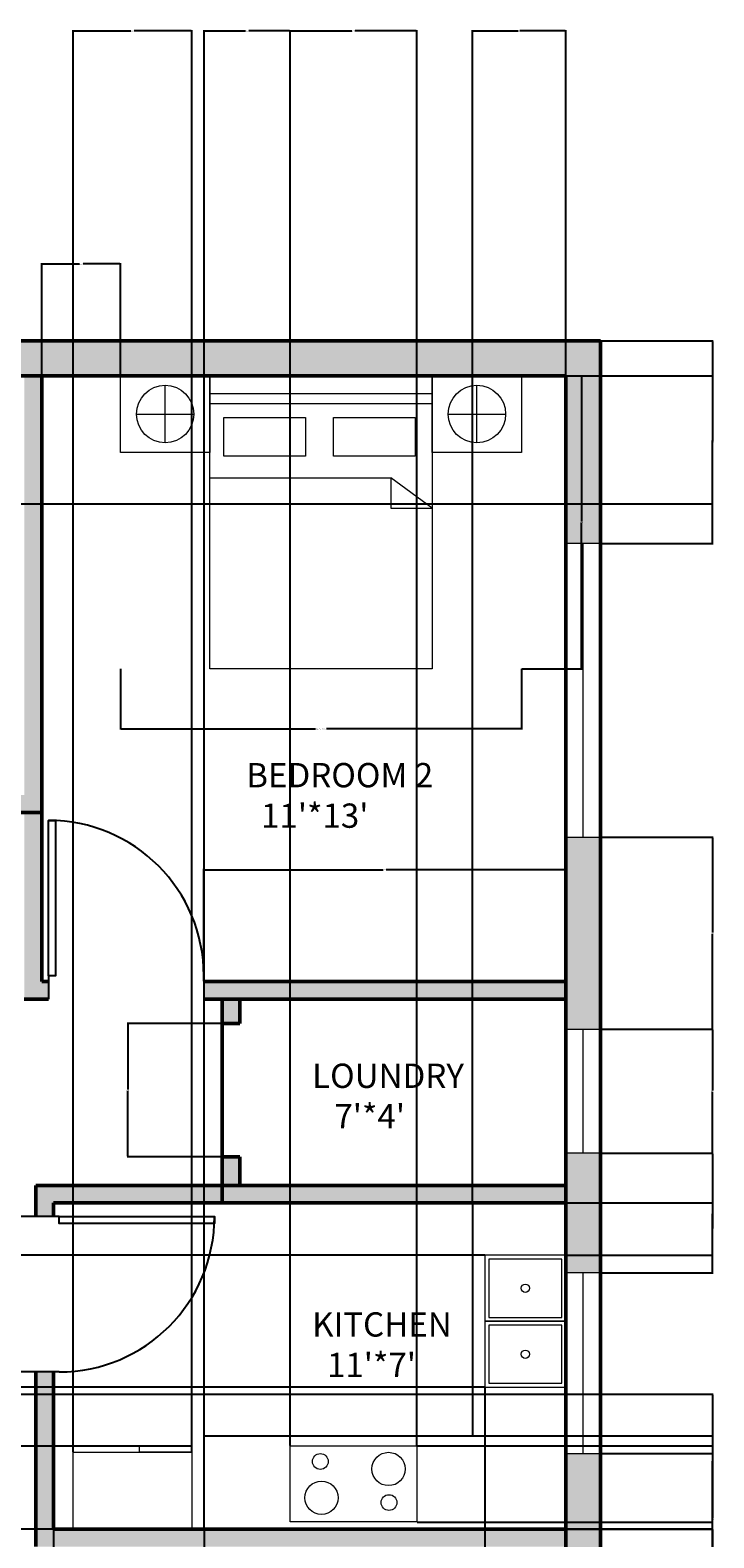
# Model space of a CAD drawing. Units: inches. Extents: x 2405 to 2823, y 1214 to 1813.
# Tile 4 of 4: x 2647 to 2823, y 1425 to 1813. Entities that reach past the tile are written whole.
import ezdxf

# ---------------------------------------------------------------- set-up
doc = ezdxf.new("R2010")
doc.units = ezdxf.units.IN
for name, color, linetype, lineweight in [('A-ANNO-DIMS', 2, 'Continuous', 18), ('A-AREA-IDEN', 30, 'Continuous', 25), ('A-EQPM', 8, 'Continuous', 18), ('A-FLOR-CASE', 8, 'Continuous', 25), ('A-FLOR-FIXT', 9, 'Continuous', 18), ('A-WALL-PATT', 252, 'Continuous', 13), ('DOOR', 133, 'Continuous', 25), ('FUR', 10, 'Continuous', 18), ('WALL', 140, 'Continuous', 50), ('WIND', 200, 'Continuous', 18)]:
    doc.layers.add(name, color=color, linetype=linetype, lineweight=lineweight)
doc.styles.get("Standard").update_dxf_attribs({"font": 'arial.ttf'})
doc.dimstyles.get("Standard").update_dxf_attribs({"dimtxt": 0.18, "dimasz": 0.18, "dimexe": 0.18, "dimexo": 0.0625, "dimgap": 0.09, "dimtad": 0, "dimtih": 1, "dimtoh": 1, "dimdec": 4, "dimzin": 0, "dimdsep": 46, "dimtxsty": 'Standard', "dimcen": 0.09, "dimadec": 0, "dimazin": 0, "dimtfac": 1, "dimtdec": 4, "dimtofl": 0, "dimtmove": 0, "dimatfit": 3, "dimfxl": 1, "dimtolj": 1, "dimtzin": 0, "dimarcsym": 0})

# ---------------------------------------------------------------- blocks, each defined once
blk = doc.blocks.new('*U2')
for p, q in [((0, 0), (0, -6)), ((40, 0), (40, -6))]:
    blk.add_line(p, q)
blk.add_lwpolyline([(0, 0), (0, 40), (1.75, 40), (1.75, 0)], close=True)
blk.add_arc((0, 0), 40, 0, 90)
blk = doc.blocks.new('BED-DOUBLE-WITH-NIGHTSTANDS')
for p, q in [((11.49, 58.17), (11.49, 72.97)), ((91.81, 58.17), (91.81, 72.97)), ((4.09, 65.57), (18.88, 65.57)), ((84.41, 65.57), (99.2, 65.57)), ((22.97, 49.14), (69.63, 49.14)), ((69.63, 49.14), (69.63, 41.32)), ((80.32, 41.32), (69.63, 49.14)), ((69.63, 41.32), (80.32, 41.32))]:
    blk.add_line(p, q)
for points in [[(0, 75.45), (22.97, 75.45), (22.97, 55.69), (0, 55.69)], [(22.97, 75.45), (80.32, 75.45), (80.32, 0), (22.97, 0)], [(80.32, 75.45), (103.29, 75.45), (103.29, 55.69), (80.32, 55.69)], [(22.97, 70.85), (80.32, 70.85), (80.32, 68.18), (22.97, 68.18)], [(26.59, 64.68), (47.64, 64.68), (47.64, 54.75), (26.59, 54.75)], [(54.85, 64.68), (75.89, 64.68), (75.89, 54.75), (54.85, 54.75)]]:
    blk.add_lwpolyline(points, close=True)
for centre in [(11.49, 65.57), (91.81, 65.57)]:
    blk.add_circle(centre, 7.4)
blk = doc.blocks.new('WIN-75_625')
blk.add_line((4.5, 0), (4.5, 75.63))
blk.add_lwpolyline([(9, 75.63), (0, 75.63), (0, 0), (9, 0)], close=True)
blk = doc.blocks.new('WIN-46_53')
blk.add_line((4.5, 0), (4.5, 46.53))
blk.add_lwpolyline([(0, 0), (9, 0), (9, 46.53), (0, 46.53)], close=True)
blk = doc.blocks.new('*D16')
at = {"layer": 'A-ANNO-DIMS', "color": 0, "lineweight": -2, "transparency": 16777216}
for p, q in [((2670.07, 1648.42), (2670.07, 1632.81)), ((2773.36, 1648.42), (2773.36, 1632.81)), ((2670.25, 1632.99), (2720.34, 1632.99)), ((2773.18, 1632.99), (2723.1, 1632.99))]:
    blk.add_line(p, q, dxfattribs=at)
at = {"layer": 'A-ANNO-DIMS', "color": 0, "lineweight": 100, "transparency": 16777216}
for points in [[(2670.25, 1633.02), (2670.25, 1632.96), (2670.07, 1632.99)], [(2773.18, 1633.02), (2773.18, 1632.96), (2773.36, 1632.99)]]:
    blk.add_solid(points, dxfattribs=at)
at = {"layer": 'Defpoints', "color": 0, "lineweight": 100, "transparency": 16777216}
for p in [(2670.07, 1648.48), (2773.36, 1648.48), (2773.36, 1632.99)]:
    blk.add_point(p, dxfattribs=at)
at = {"layer": 'A-ANNO-DIMS', "color": 0, "transparency": 16777216, "insert": (2721.72, 1632.99), "char_height": 0.18, "attachment_point": 5}
blk.add_mtext('\\A1;BED GROUP 103 TYP.', dxfattribs=at)
blk = doc.blocks.new('*D17')
at = {"layer": 'A-ANNO-DIMS', "color": 0, "lineweight": -2, "transparency": 16777216}
for p, q in [((2773.43, 1723.93), (2789.04, 1723.93)), ((2788.86, 1723.75), (2788.86, 1686.39)), ((2788.86, 1648.66), (2788.86, 1686.02)), ((2773.43, 1648.48), (2789.04, 1648.48))]:
    blk.add_line(p, q, dxfattribs=at)
at = {"layer": 'A-ANNO-DIMS', "color": 0, "lineweight": 100, "transparency": 16777216}
for points in [[(2788.83, 1723.75), (2788.89, 1723.75), (2788.86, 1723.93)], [(2788.83, 1648.66), (2788.89, 1648.66), (2788.86, 1648.48)]]:
    blk.add_solid(points, dxfattribs=at)
at = {"layer": 'Defpoints', "color": 0, "lineweight": 100, "transparency": 16777216}
for p in [(2773.36, 1723.93), (2788.86, 1723.93), (2773.36, 1648.48)]:
    blk.add_point(p, dxfattribs=at)
at = {"layer": 'A-ANNO-DIMS', "color": 0, "transparency": 16777216, "insert": (2788.86, 1686.21), "char_height": 0.18, "attachment_point": 5}
blk.add_mtext('\\A1;75 TYP.', dxfattribs=at)
blk = doc.blocks.new('*D24')
at = {"layer": 'A-ANNO-DIMS', "color": 0, "lineweight": -2, "transparency": 16777216}
for p, q in [((2793.83, 1732.93), (2822.75, 1732.93)), ((2822.57, 1732.75), (2822.57, 1707.02)), ((2822.57, 1680.92), (2822.57, 1706.65)), ((2793.83, 1680.74), (2822.75, 1680.74))]:
    blk.add_line(p, q, dxfattribs=at)
at = {"layer": 'A-ANNO-DIMS', "color": 0, "lineweight": 100, "transparency": 16777216}
for points in [[(2822.54, 1732.75), (2822.6, 1732.75), (2822.57, 1732.93)], [(2822.54, 1680.92), (2822.6, 1680.92), (2822.57, 1680.74)]]:
    blk.add_solid(points, dxfattribs=at)
at = {"layer": 'Defpoints', "color": 0, "lineweight": 100, "transparency": 16777216}
for p in [(2793.77, 1732.93), (2793.77, 1680.74), (2822.57, 1680.74)]:
    blk.add_point(p, dxfattribs=at)
at = {"layer": 'A-ANNO-DIMS', "color": 0, "transparency": 16777216, "insert": (2822.57, 1706.83), "char_height": 0.18, "attachment_point": 5}
blk.add_mtext('\\A1;52.19', dxfattribs=at)
blk = doc.blocks.new('*D26')
at = {"layer": 'A-ANNO-DIMS', "color": 0, "lineweight": -2, "transparency": 16777216}
for p, q in [((2793.83, 1605.11), (2822.75, 1605.11)), ((2822.57, 1604.93), (2822.57, 1580.57)), ((2822.57, 1555.85), (2822.57, 1580.21)), ((2793.83, 1555.67), (2822.75, 1555.67))]:
    blk.add_line(p, q, dxfattribs=at)
at = {"layer": 'A-ANNO-DIMS', "color": 0, "lineweight": 100, "transparency": 16777216}
for points in [[(2822.54, 1604.93), (2822.6, 1604.93), (2822.57, 1605.11)], [(2822.54, 1555.85), (2822.6, 1555.85), (2822.57, 1555.67)]]:
    blk.add_solid(points, dxfattribs=at)
at = {"layer": 'Defpoints', "color": 0, "lineweight": 100, "transparency": 16777216}
for p in [(2793.77, 1605.11), (2793.77, 1555.67), (2822.57, 1555.67)]:
    blk.add_point(p, dxfattribs=at)
at = {"layer": 'A-ANNO-DIMS', "color": 0, "transparency": 16777216, "insert": (2822.57, 1580.39), "char_height": 0.18, "attachment_point": 5}
blk.add_mtext('\\A1;49.44', dxfattribs=at)
blk = doc.blocks.new('*D27')
at = {"layer": 'A-ANNO-DIMS', "color": 0, "lineweight": -2, "transparency": 16777216}
for p, q in [((2793.83, 1555.67), (2822.75, 1555.67)), ((2822.57, 1555.49), (2822.57, 1539.88)), ((2822.57, 1523.92), (2822.57, 1539.52)), ((2793.83, 1523.74), (2822.75, 1523.74))]:
    blk.add_line(p, q, dxfattribs=at)
at = {"layer": 'A-ANNO-DIMS', "color": 0, "lineweight": 100, "transparency": 16777216}
for points in [[(2822.54, 1555.49), (2822.6, 1555.49), (2822.57, 1555.67)], [(2822.54, 1523.92), (2822.6, 1523.92), (2822.57, 1523.74)]]:
    blk.add_solid(points, dxfattribs=at)
at = {"layer": 'Defpoints', "color": 0, "lineweight": 100, "transparency": 16777216}
for p in [(2793.77, 1555.67), (2793.77, 1523.74), (2822.57, 1523.74)]:
    blk.add_point(p, dxfattribs=at)
at = {"layer": 'A-ANNO-DIMS', "color": 0, "transparency": 16777216, "insert": (2822.57, 1539.7), "char_height": 0.18, "attachment_point": 5}
blk.add_mtext('\\A1;31.93', dxfattribs=at)
blk = doc.blocks.new('*D28')
at = {"layer": 'A-ANNO-DIMS', "color": 0, "lineweight": -2, "transparency": 16777216}
for p, q in [((2793.83, 1523.74), (2822.75, 1523.74)), ((2822.57, 1523.56), (2822.57, 1508.52)), ((2822.57, 1493.11), (2822.57, 1508.15)), ((2793.83, 1492.93), (2822.75, 1492.93))]:
    blk.add_line(p, q, dxfattribs=at)
at = {"layer": 'A-ANNO-DIMS', "color": 0, "lineweight": 100, "transparency": 16777216}
for points in [[(2822.54, 1523.56), (2822.6, 1523.56), (2822.57, 1523.74)], [(2822.54, 1493.11), (2822.6, 1493.11), (2822.57, 1492.93)]]:
    blk.add_solid(points, dxfattribs=at)
at = {"layer": 'Defpoints', "color": 0, "lineweight": 100, "transparency": 16777216}
for p in [(2793.77, 1523.74), (2793.77, 1492.93), (2822.57, 1492.93)]:
    blk.add_point(p, dxfattribs=at)
at = {"layer": 'A-ANNO-DIMS', "color": 0, "transparency": 16777216, "insert": (2822.57, 1508.33), "char_height": 0.18, "attachment_point": 5}
blk.add_mtext('\\A1;30.807', dxfattribs=at)
blk = doc.blocks.new('*D29')
at = {"layer": 'A-ANNO-DIMS', "color": 0, "lineweight": -2, "transparency": 16777216}
for p, q in [((2793.83, 1446.4), (2822.75, 1446.4)), ((2822.57, 1446.22), (2822.57, 1429.71)), ((2822.57, 1412.83), (2822.57, 1429.35)), ((2793.83, 1412.65), (2822.75, 1412.65))]:
    blk.add_line(p, q, dxfattribs=at)
at = {"layer": 'A-ANNO-DIMS', "color": 0, "lineweight": 100, "transparency": 16777216}
for points in [[(2822.54, 1446.22), (2822.6, 1446.22), (2822.57, 1446.4)], [(2822.54, 1412.83), (2822.6, 1412.83), (2822.57, 1412.65)]]:
    blk.add_solid(points, dxfattribs=at)
at = {"layer": 'Defpoints', "color": 0, "lineweight": 100, "transparency": 16777216}
for p in [(2793.77, 1446.4), (2793.77, 1412.65), (2822.57, 1412.65)]:
    blk.add_point(p, dxfattribs=at)
at = {"layer": 'A-ANNO-DIMS', "color": 0, "transparency": 16777216, "insert": (2822.57, 1429.53), "char_height": 0.18, "attachment_point": 5}
blk.add_mtext('\\A1;33.754', dxfattribs=at)
blk = doc.blocks.new('*D38')
at = {"layer": 'A-ANNO-DIMS', "color": 0, "lineweight": -2, "transparency": 16777216}
for p, q in [((2760.77, 1510.99), (2760.77, 1812.91)), ((2760.95, 1812.73), (2772.55, 1812.73)), ((2784.59, 1812.73), (2772.99, 1812.73)), ((2784.77, 1510.99), (2784.77, 1812.91))]:
    blk.add_line(p, q, dxfattribs=at)
at = {"layer": 'A-ANNO-DIMS', "color": 0, "lineweight": 100, "transparency": 16777216}
for points in [[(2760.95, 1812.76), (2760.95, 1812.7), (2760.77, 1812.73)], [(2784.59, 1812.76), (2784.59, 1812.7), (2784.77, 1812.73)]]:
    blk.add_solid(points, dxfattribs=at)
at = {"layer": 'Defpoints', "color": 0, "lineweight": 100, "transparency": 16777216}
for p in [(2760.77, 1812.73), (2760.77, 1510.93), (2784.77, 1510.93)]:
    blk.add_point(p, dxfattribs=at)
at = {"layer": 'A-ANNO-DIMS', "color": 0, "transparency": 16777216, "insert": (2772.77, 1812.73), "char_height": 0.18, "attachment_point": 5}
blk.add_mtext('\\A1;24', dxfattribs=at)
blk = doc.blocks.new('*D39')
at = {"layer": 'A-ANNO-DIMS', "color": 0, "lineweight": -2, "transparency": 16777216}
for p, q in [((2691.69, 1450.93), (2822.75, 1450.93)), ((2822.57, 1450.75), (2822.57, 1439.11)), ((2822.57, 1427.11), (2822.57, 1438.75)), ((2691.69, 1426.93), (2822.75, 1426.93))]:
    blk.add_line(p, q, dxfattribs=at)
at = {"layer": 'A-ANNO-DIMS', "color": 0, "lineweight": 100, "transparency": 16777216}
for points in [[(2822.54, 1450.75), (2822.6, 1450.75), (2822.57, 1450.93)], [(2822.54, 1427.11), (2822.6, 1427.11), (2822.57, 1426.93)]]:
    blk.add_solid(points, dxfattribs=at)
at = {"layer": 'Defpoints', "color": 0, "lineweight": 100, "transparency": 16777216}
for p in [(2691.63, 1450.93), (2691.63, 1426.93), (2822.57, 1426.93)]:
    blk.add_point(p, dxfattribs=at)
at = {"layer": 'A-ANNO-DIMS', "color": 0, "transparency": 16777216, "insert": (2822.57, 1438.93), "char_height": 0.18, "attachment_point": 5}
blk.add_mtext('\\A1;24', dxfattribs=at)
blk = doc.blocks.new('*D40')
at = {"layer": 'A-ANNO-DIMS', "color": 0, "lineweight": -2, "transparency": 16777216}
for p, q in [((2652.77, 1426.87), (2652.77, 1214.95)), ((2691.63, 1426.87), (2691.63, 1214.95)), ((2652.95, 1215.13), (2671.8, 1215.13)), ((2691.45, 1215.13), (2672.59, 1215.13))]:
    blk.add_line(p, q, dxfattribs=at)
at = {"layer": 'A-ANNO-DIMS', "color": 0, "lineweight": 100, "transparency": 16777216}
for points in [[(2652.95, 1215.16), (2652.95, 1215.1), (2652.77, 1215.13)], [(2691.45, 1215.16), (2691.45, 1215.1), (2691.63, 1215.13)]]:
    blk.add_solid(points, dxfattribs=at)
at = {"layer": 'Defpoints', "color": 0, "lineweight": 100, "transparency": 16777216}
for p in [(2652.77, 1426.93), (2691.63, 1426.93), (2691.63, 1215.13)]:
    blk.add_point(p, dxfattribs=at)
at = {"layer": 'A-ANNO-DIMS', "color": 0, "transparency": 16777216, "insert": (2672.2, 1215.13), "char_height": 0.18, "attachment_point": 5}
blk.add_mtext('\\A1;38.86', dxfattribs=at)
blk = doc.blocks.new('*D41')
at = {"layer": 'A-ANNO-DIMS', "color": 0, "lineweight": -2, "transparency": 16777216}
for p, q in [((2648.21, 1507.39), (2404.79, 1507.39)), ((2404.97, 1507.21), (2404.97, 1487.57)), ((2404.97, 1467.57), (2404.97, 1487.21)), ((2648.21, 1467.39), (2404.79, 1467.39))]:
    blk.add_line(p, q, dxfattribs=at)
at = {"layer": 'A-ANNO-DIMS', "color": 0, "lineweight": 100, "transparency": 16777216}
for points in [[(2404.94, 1507.21), (2405, 1507.21), (2404.97, 1507.39)], [(2404.94, 1467.57), (2405, 1467.57), (2404.97, 1467.39)]]:
    blk.add_solid(points, dxfattribs=at)
at = {"layer": 'Defpoints', "color": 0, "lineweight": 100, "transparency": 16777216}
for p in [(2648.27, 1507.39), (2404.97, 1467.39), (2648.27, 1467.39)]:
    blk.add_point(p, dxfattribs=at)
at = {"layer": 'A-ANNO-DIMS', "color": 0, "transparency": 16777216, "insert": (2404.97, 1487.39), "char_height": 0.18, "attachment_point": 5}
blk.add_mtext('\\A1;40', dxfattribs=at)
blk = doc.blocks.new('*D45')
at = {"layer": 'A-ANNO-DIMS', "color": 0, "lineweight": -2, "transparency": 16777216}
for p, q in [((2477.36, 1461.68), (2822.75, 1461.68)), ((2822.57, 1461.5), (2822.57, 1444.53)), ((2822.57, 1427.19), (2822.57, 1444.16)), ((2477.36, 1427.01), (2822.75, 1427.01))]:
    blk.add_line(p, q, dxfattribs=at)
at = {"layer": 'A-ANNO-DIMS', "color": 0, "lineweight": 100, "transparency": 16777216}
for points in [[(2822.54, 1461.5), (2822.6, 1461.5), (2822.57, 1461.68)], [(2822.54, 1427.19), (2822.6, 1427.19), (2822.57, 1427.01)]]:
    blk.add_solid(points, dxfattribs=at)
at = {"layer": 'Defpoints', "color": 0, "lineweight": 100, "transparency": 16777216}
for p in [(2477.3, 1461.68), (2477.3, 1427.01), (2822.57, 1427.01)]:
    blk.add_point(p, dxfattribs=at)
at = {"layer": 'A-ANNO-DIMS', "color": 0, "transparency": 16777216, "insert": (2822.57, 1444.34), "char_height": 0.18, "attachment_point": 5}
blk.add_mtext('\\A1;34.66', dxfattribs=at)
blk = doc.blocks.new('*D46')
at = {"layer": 'A-ANNO-DIMS', "color": 0, "lineweight": -2, "transparency": 16777216}
for p, q in [((2713.75, 1448.42), (2713.75, 1812.91)), ((2713.93, 1812.73), (2729.63, 1812.73)), ((2746.25, 1812.73), (2730.56, 1812.73)), ((2746.43, 1448.42), (2746.43, 1812.91))]:
    blk.add_line(p, q, dxfattribs=at)
at = {"layer": 'A-ANNO-DIMS', "color": 0, "lineweight": 100, "transparency": 16777216}
for points in [[(2713.93, 1812.76), (2713.93, 1812.7), (2713.75, 1812.73)], [(2746.25, 1812.76), (2746.25, 1812.7), (2746.43, 1812.73)]]:
    blk.add_solid(points, dxfattribs=at)
at = {"layer": 'Defpoints', "color": 0, "lineweight": 100, "transparency": 16777216}
for p in [(2746.43, 1812.73), (2713.75, 1448.36), (2746.43, 1448.36)]:
    blk.add_point(p, dxfattribs=at)
at = {"layer": 'A-ANNO-DIMS', "color": 0, "transparency": 16777216, "insert": (2730.09, 1812.73), "char_height": 0.18, "attachment_point": 5}
blk.add_mtext('\\A1;32.684', dxfattribs=at)
blk = doc.blocks.new('*D47')
at = {"layer": 'A-ANNO-DIMS', "color": 0, "lineweight": -2, "transparency": 16777216}
for p, q in [((2763.89, 1497.45), (2404.79, 1497.45)), ((2404.97, 1497.27), (2404.97, 1480.64)), ((2404.97, 1463.65), (2404.97, 1480.28)), ((2763.89, 1463.47), (2404.79, 1463.47))]:
    blk.add_line(p, q, dxfattribs=at)
at = {"layer": 'A-ANNO-DIMS', "color": 0, "lineweight": 100, "transparency": 16777216}
for points in [[(2404.94, 1497.27), (2405, 1497.27), (2404.97, 1497.45)], [(2404.94, 1463.65), (2405, 1463.65), (2404.97, 1463.47)]]:
    blk.add_solid(points, dxfattribs=at)
at = {"layer": 'Defpoints', "color": 0, "lineweight": 100, "transparency": 16777216}
for p in [(2763.95, 1497.45), (2404.97, 1463.47), (2763.95, 1463.47)]:
    blk.add_point(p, dxfattribs=at)
at = {"layer": 'A-ANNO-DIMS', "color": 0, "transparency": 16777216, "insert": (2404.97, 1480.46), "char_height": 0.18, "attachment_point": 5}
blk.add_mtext('\\A1;33.98', dxfattribs=at)
blk = doc.blocks.new('*D48')
at = {"layer": 'A-ANNO-DIMS', "color": 0, "lineweight": -2, "transparency": 16777216}
for p, q in [((2763.95, 1463.41), (2763.95, 1214.95)), ((2784.77, 1463.41), (2784.77, 1214.95)), ((2764.13, 1215.13), (2773.9, 1215.13)), ((2784.59, 1215.13), (2774.83, 1215.13))]:
    blk.add_line(p, q, dxfattribs=at)
at = {"layer": 'A-ANNO-DIMS', "color": 0, "lineweight": 100, "transparency": 16777216}
for points in [[(2764.13, 1215.16), (2764.13, 1215.1), (2763.95, 1215.13)], [(2784.59, 1215.16), (2784.59, 1215.1), (2784.77, 1215.13)]]:
    blk.add_solid(points, dxfattribs=at)
at = {"layer": 'Defpoints', "color": 0, "lineweight": 100, "transparency": 16777216}
for p in [(2763.95, 1463.47), (2784.77, 1463.47), (2784.77, 1215.13)]:
    blk.add_point(p, dxfattribs=at)
at = {"layer": 'A-ANNO-DIMS', "color": 0, "transparency": 16777216, "insert": (2774.36, 1215.13), "char_height": 0.18, "attachment_point": 5}
blk.add_mtext('\\A1;20.813', dxfattribs=at)
blk = doc.blocks.new('*D50')
at = {"layer": 'A-ANNO-DIMS', "color": 0, "lineweight": -2, "transparency": 16777216}
for p, q in [((2477.36, 1427.01), (2822.75, 1427.01)), ((2822.57, 1426.83), (2822.57, 1414.4)), ((2822.57, 1401.61), (2822.57, 1414.04)), ((2442.83, 1401.43), (2822.75, 1401.43))]:
    blk.add_line(p, q, dxfattribs=at)
at = {"layer": 'A-ANNO-DIMS', "color": 0, "lineweight": 100, "transparency": 16777216}
for points in [[(2822.54, 1426.83), (2822.6, 1426.83), (2822.57, 1427.01)], [(2822.54, 1401.61), (2822.6, 1401.61), (2822.57, 1401.43)]]:
    blk.add_solid(points, dxfattribs=at)
at = {"layer": 'Defpoints', "color": 0, "lineweight": 100, "transparency": 16777216}
for p in [(2477.3, 1427.01), (2822.57, 1427.01), (2442.77, 1401.43)]:
    blk.add_point(p, dxfattribs=at)
at = {"layer": 'A-ANNO-DIMS', "color": 0, "transparency": 16777216, "insert": (2822.57, 1414.22), "char_height": 0.18, "attachment_point": 5}
blk.add_mtext('\\A1;25.584', dxfattribs=at)
blk = doc.blocks.new('*D51')
at = {"layer": 'A-ANNO-DIMS', "color": 0, "lineweight": -2, "transparency": 16777216}
for p, q in [((2746.5, 1448.36), (2822.75, 1448.36)), ((2822.57, 1448.18), (2822.57, 1438.74)), ((2822.57, 1428.94), (2822.57, 1438.38)), ((2746.5, 1428.76), (2822.75, 1428.76))]:
    blk.add_line(p, q, dxfattribs=at)
at = {"layer": 'A-ANNO-DIMS', "color": 0, "lineweight": 100, "transparency": 16777216}
for points in [[(2822.54, 1448.18), (2822.6, 1448.18), (2822.57, 1448.36)], [(2822.54, 1428.94), (2822.6, 1428.94), (2822.57, 1428.76)]]:
    blk.add_solid(points, dxfattribs=at)
at = {"layer": 'Defpoints', "color": 0, "lineweight": 100, "transparency": 16777216}
for p in [(2746.43, 1448.36), (2746.43, 1428.76), (2822.57, 1428.76)]:
    blk.add_point(p, dxfattribs=at)
at = {"layer": 'A-ANNO-DIMS', "color": 0, "transparency": 16777216, "insert": (2822.57, 1438.56), "char_height": 0.18, "attachment_point": 5}
blk.add_mtext('\\A1;19.593', dxfattribs=at)
blk = doc.blocks.new('*D53')
at = {"layer": 'A-ANNO-DIMS', "color": 0, "lineweight": -2, "transparency": 16777216}
for p, q in [((2649.77, 1723.99), (2649.77, 1752.91)), ((2649.95, 1752.73), (2659.45, 1752.73)), ((2669.89, 1752.73), (2660.39, 1752.73)), ((2670.07, 1723.99), (2670.07, 1752.91))]:
    blk.add_line(p, q, dxfattribs=at)
at = {"layer": 'A-ANNO-DIMS', "color": 0, "lineweight": 100, "transparency": 16777216}
for points in [[(2649.95, 1752.76), (2649.95, 1752.7), (2649.77, 1752.73)], [(2669.89, 1752.76), (2669.89, 1752.7), (2670.07, 1752.73)]]:
    blk.add_solid(points, dxfattribs=at)
at = {"layer": 'Defpoints', "color": 0, "lineweight": 100, "transparency": 16777216}
for p in [(2670.07, 1752.73), (2649.77, 1723.93), (2670.07, 1723.93)]:
    blk.add_point(p, dxfattribs=at)
at = {"layer": 'A-ANNO-DIMS', "color": 0, "transparency": 16777216, "insert": (2659.92, 1752.73), "char_height": 0.18, "attachment_point": 5}
blk.add_mtext('\\A1;20.305', dxfattribs=at)
blk = doc.blocks.new('*D55')
at = {"layer": 'A-ANNO-DIMS', "color": 0, "lineweight": -2, "transparency": 16777216}
for p, q in [((2700.71, 1557.1), (2671.79, 1557.1)), ((2671.97, 1556.92), (2671.97, 1540.13)), ((2671.97, 1522.97), (2671.97, 1539.77)), ((2700.71, 1522.79), (2671.79, 1522.79))]:
    blk.add_line(p, q, dxfattribs=at)
at = {"layer": 'A-ANNO-DIMS', "color": 0, "lineweight": 100, "transparency": 16777216}
for points in [[(2671.94, 1556.92), (2672, 1556.92), (2671.97, 1557.1)], [(2671.94, 1522.97), (2672, 1522.97), (2671.97, 1522.79)]]:
    blk.add_solid(points, dxfattribs=at)
at = {"layer": 'Defpoints', "color": 0, "lineweight": 100, "transparency": 16777216}
for p in [(2671.97, 1557.1), (2700.77, 1557.1), (2700.77, 1522.79)]:
    blk.add_point(p, dxfattribs=at)
at = {"layer": 'A-ANNO-DIMS', "color": 0, "transparency": 16777216, "insert": (2671.97, 1539.95), "char_height": 0.18, "attachment_point": 5}
blk.add_mtext('\\A1;34.31', dxfattribs=at)
blk = doc.blocks.new('*D57')
at = {"layer": 'A-ANNO-DIMS', "color": 0, "lineweight": -2, "transparency": 16777216}
for p, q in [((2622.83, 1723.93), (2822.75, 1723.93)), ((2822.57, 1723.75), (2822.57, 1707.61)), ((2822.57, 1691.11), (2822.57, 1707.25)), ((2612.33, 1690.93), (2822.75, 1690.93))]:
    blk.add_line(p, q, dxfattribs=at)
at = {"layer": 'A-ANNO-DIMS', "color": 0, "lineweight": 100, "transparency": 16777216}
for points in [[(2822.54, 1723.75), (2822.6, 1723.75), (2822.57, 1723.93)], [(2822.54, 1691.11), (2822.6, 1691.11), (2822.57, 1690.93)]]:
    blk.add_solid(points, dxfattribs=at)
at = {"layer": 'Defpoints', "color": 0, "lineweight": 100, "transparency": 16777216}
for p in [(2622.77, 1723.93), (2612.27, 1690.93), (2822.57, 1690.93)]:
    blk.add_point(p, dxfattribs=at)
at = {"layer": 'A-ANNO-DIMS', "color": 0, "transparency": 16777216, "insert": (2822.57, 1707.43), "char_height": 0.18, "attachment_point": 5}
blk.add_mtext('\\A1;33', dxfattribs=at)
blk = doc.blocks.new('*D58')
at = {"layer": 'A-ANNO-DIMS', "color": 0, "lineweight": -2, "transparency": 16777216}
for p, q in [((2691.63, 1450.99), (2691.63, 1812.91)), ((2691.81, 1812.73), (2702.3, 1812.73)), ((2713.57, 1812.73), (2703.08, 1812.73)), ((2713.75, 1448.42), (2713.75, 1812.91))]:
    blk.add_line(p, q, dxfattribs=at)
at = {"layer": 'A-ANNO-DIMS', "color": 0, "lineweight": 100, "transparency": 16777216}
for points in [[(2691.81, 1812.76), (2691.81, 1812.7), (2691.63, 1812.73)], [(2713.57, 1812.76), (2713.57, 1812.7), (2713.75, 1812.73)]]:
    blk.add_solid(points, dxfattribs=at)
at = {"layer": 'Defpoints', "color": 0, "lineweight": 100, "transparency": 16777216}
for p in [(2713.75, 1812.73), (2691.63, 1450.93), (2713.75, 1448.36)]:
    blk.add_point(p, dxfattribs=at)
at = {"layer": 'A-ANNO-DIMS', "color": 0, "transparency": 16777216, "insert": (2702.69, 1812.73), "char_height": 0.18, "attachment_point": 5}
blk.add_mtext('\\A1;22.12', dxfattribs=at)
blk = doc.blocks.new('*D59')
at = {"layer": 'A-ANNO-DIMS', "color": 0, "lineweight": -2, "transparency": 16777216}
for p, q in [((2784.83, 1510.93), (2822.75, 1510.93)), ((2822.57, 1510.75), (2822.57, 1504.37)), ((2822.57, 1497.63), (2822.57, 1504.01)), ((2784.83, 1497.45), (2822.75, 1497.45))]:
    blk.add_line(p, q, dxfattribs=at)
at = {"layer": 'A-ANNO-DIMS', "color": 0, "lineweight": 100, "transparency": 16777216}
for points in [[(2822.54, 1510.75), (2822.6, 1510.75), (2822.57, 1510.93)], [(2822.54, 1497.63), (2822.6, 1497.63), (2822.57, 1497.45)]]:
    blk.add_solid(points, dxfattribs=at)
at = {"layer": 'Defpoints', "color": 0, "lineweight": 100, "transparency": 16777216}
for p in [(2784.77, 1510.93), (2822.57, 1510.93), (2784.77, 1497.45)]:
    blk.add_point(p, dxfattribs=at)
at = {"layer": 'A-ANNO-DIMS', "color": 0, "transparency": 16777216, "insert": (2822.57, 1504.19), "char_height": 0.18, "attachment_point": 5}
blk.add_mtext('\\A1;13.477', dxfattribs=at)
blk = doc.blocks.new('*D66')
at = {"layer": 'A-ANNO-DIMS', "color": 0, "lineweight": -2, "transparency": 16777216}
for p, q in [((2691.52, 1567.99), (2691.52, 1596.91)), ((2691.7, 1596.73), (2737.75, 1596.73)), ((2784.59, 1596.73), (2738.54, 1596.73)), ((2784.77, 1567.99), (2784.77, 1596.91))]:
    blk.add_line(p, q, dxfattribs=at)
at = {"layer": 'A-ANNO-DIMS', "color": 0, "lineweight": 100, "transparency": 16777216}
for points in [[(2691.7, 1596.76), (2691.7, 1596.7), (2691.52, 1596.73)], [(2784.59, 1596.76), (2784.59, 1596.7), (2784.77, 1596.73)]]:
    blk.add_solid(points, dxfattribs=at)
at = {"layer": 'Defpoints', "color": 0, "lineweight": 100, "transparency": 16777216}
for p in [(2784.77, 1596.73), (2691.52, 1567.93), (2784.77, 1567.93)]:
    blk.add_point(p, dxfattribs=at)
at = {"layer": 'A-ANNO-DIMS', "color": 0, "transparency": 16777216, "insert": (2738.14, 1596.73), "char_height": 0.18, "attachment_point": 5}
blk.add_mtext('\\A1;93.25', dxfattribs=at)
blk = doc.blocks.new('*D67')
at = {"layer": 'A-ANNO-DIMS', "color": 0, "lineweight": -2, "transparency": 16777216}
for p, q in [((2657.86, 1446.84), (2657.86, 1812.91)), ((2658.04, 1812.73), (2672.68, 1812.73)), ((2688.24, 1812.73), (2673.6, 1812.73)), ((2688.42, 1446.84), (2688.42, 1812.91))]:
    blk.add_line(p, q, dxfattribs=at)
at = {"layer": 'A-ANNO-DIMS', "color": 0, "lineweight": 100, "transparency": 16777216}
for points in [[(2658.04, 1812.76), (2658.04, 1812.7), (2657.86, 1812.73)], [(2688.24, 1812.76), (2688.24, 1812.7), (2688.42, 1812.73)]]:
    blk.add_solid(points, dxfattribs=at)
at = {"layer": 'Defpoints', "color": 0, "lineweight": 100, "transparency": 16777216}
for p in [(2688.42, 1812.73), (2657.86, 1446.78), (2688.42, 1446.78)]:
    blk.add_point(p, dxfattribs=at)
at = {"layer": 'A-ANNO-DIMS', "color": 0, "transparency": 16777216, "insert": (2673.14, 1812.73), "char_height": 0.18, "attachment_point": 5}
blk.add_mtext('\\A1;30.564', dxfattribs=at)
blk = doc.blocks.new('*D68')
at = {"layer": 'A-ANNO-DIMS', "color": 0, "lineweight": -2, "transparency": 16777216}
for p, q in [((2688.36, 1448.27), (2404.79, 1448.27)), ((2404.97, 1448.09), (2404.97, 1437.78)), ((2404.97, 1427.11), (2404.97, 1437.42)), ((2688.36, 1426.93), (2404.79, 1426.93))]:
    blk.add_line(p, q, dxfattribs=at)
at = {"layer": 'A-ANNO-DIMS', "color": 0, "lineweight": 100, "transparency": 16777216}
for points in [[(2404.94, 1448.09), (2405, 1448.09), (2404.97, 1448.27)], [(2404.94, 1427.11), (2405, 1427.11), (2404.97, 1426.93)]]:
    blk.add_solid(points, dxfattribs=at)
at = {"layer": 'Defpoints', "color": 0, "lineweight": 100, "transparency": 16777216}
for p in [(2688.42, 1448.27), (2404.97, 1426.93), (2688.42, 1426.93)]:
    blk.add_point(p, dxfattribs=at)
at = {"layer": 'A-ANNO-DIMS', "color": 0, "transparency": 16777216, "insert": (2404.97, 1437.6), "char_height": 0.18, "attachment_point": 5}
blk.add_mtext('\\A1;21.336', dxfattribs=at)

msp = doc.modelspace()

# ---------------------------------------------------------------- hatches: boundary and pattern name
at = {"layer": 'A-WALL-PATT'}
h = msp.add_hatch(color=256, dxfattribs=at)
h.dxf.hatch_style = 1
h.paths.add_polyline_path([(2601.7679, 1732.9303), (2433.7679, 1732.9303), (2433.7679, 1680.7368), (2442.7679, 1680.7368), (2442.7679, 1723.9303), (2574.7679, 1723.9303), (2601.7679, 1723.9303)])
h.paths.add_polyline_path([(2793.7679, 1732.9303), (2622.7552, 1732.9303), (2622.7552, 1723.9303), (2622.7679, 1723.9303), (2645.2679, 1723.9303), (2784.7679, 1723.9303), (2784.7679, 1680.7368), (2793.7679, 1680.7368)])
h.paths.add_polyline_path([(2442.7679, 1605.111), (2433.7679, 1605.111), (2433.7679, 1513.1454), (2442.7679, 1513.1454), (2442.7679, 1563.4303)])
h.paths.add_polyline_path([(2531.8067, 1567.9303), (2442.7679, 1567.9303), (2442.7679, 1563.4303), (2531.8067, 1563.4303)])
h.paths.add_polyline_path([(2793.7679, 1605.111), (2784.7679, 1605.111), (2784.7679, 1555.6662), (2793.7679, 1555.6662)])
h.paths.add_polyline_path([(2784.7679, 1567.9303), (2691.5187, 1567.9303), (2691.5187, 1563.4303), (2784.7679, 1563.4303)])
h.paths.add_polyline_path([(2649.7679, 1611.4303), (2645.2679, 1611.4303), (2645.2679, 1563.4303), (2651.5187, 1563.4303), (2651.5187, 1567.9303), (2649.7679, 1567.9303)])
h.paths.add_polyline_path([(2581.5295, 1614.9584), (2581.5295, 1615.9303), (2579.2679, 1615.9303), (2579.2679, 1611.4303), (2581.5295, 1611.4303)])
h.paths.add_polyline_path([(2579.2679, 1723.9303), (2574.7679, 1723.9303), (2574.7679, 1567.9303), (2571.8067, 1567.9303), (2571.8067, 1563.4303), (2579.2679, 1563.4303)])
h.paths.add_polyline_path([(2649.7679, 1723.9303), (2645.2679, 1723.9303), (2645.2679, 1615.9303), (2605.0298, 1615.9303, -0.01033406), (2605.0499, 1614.9584), (2605.0499, 1611.4303), (2649.7679, 1611.4303)])
h.paths.add_polyline_path([(2793.7679, 1523.737), (2784.7679, 1523.737), (2784.7679, 1492.9303), (2793.7679, 1492.9303)])
h.paths.add_polyline_path([(2793.7679, 1446.4039), (2784.7679, 1446.4039), (2784.7679, 1426.9303), (2784.7679, 1412.6503), (2793.7679, 1412.6503)])
h.paths.add_polyline_path([(2652.7679, 1467.3906), (2648.2679, 1467.3906), (2648.2679, 1422.4303), (2784.7679, 1422.4303), (2784.7679, 1426.9303), (2652.7679, 1426.9303)])
h.paths.add_polyline_path([(2696.2679, 1515.4303), (2648.2679, 1515.4303), (2648.2679, 1507.3906), (2652.7679, 1507.3906), (2652.7679, 1510.9303), (2696.2679, 1510.9303)])
h.paths.add_polyline_path([(2784.7679, 1515.4303), (2700.7679, 1515.4303), (2696.2679, 1515.4303), (2696.2679, 1510.9303), (2784.7679, 1510.9303)])
h.paths.add_polyline_path([(2700.7679, 1522.7934), (2696.2679, 1522.7934), (2696.2679, 1515.4303), (2700.7679, 1515.4303)])
h.paths.add_polyline_path([(2700.7679, 1563.4303), (2696.2679, 1563.4303), (2696.2679, 1557.1044), (2700.7679, 1557.1044)])
h.paths.add_polyline_path([(2442.7679, 1437.5196), (2433.7679, 1437.5196), (2433.7679, 1252.9303), (2481.6786, 1252.9303), (2481.6786, 1261.9303), (2442.7679, 1261.9303)])
h.paths.add_polyline_path([(2536.0913, 1401.4303), (2442.7679, 1401.4303), (2442.7679, 1396.9303), (2536.0913, 1396.9303)])
h.paths.add_polyline_path([(2784.7679, 1358.4303), (2630.4061, 1358.4303), (2630.4061, 1353.9303), (2784.7679, 1353.9303)])
h.paths.add_polyline_path([(2793.7679, 1366.1239), (2784.7679, 1366.1239), (2784.7679, 1261.9303), (2784.7679, 1243.9303), (2793.7679, 1243.9303), (2793.7679, 1260.2097)])
h.paths.add_polyline_path([(2590.4061, 1358.4303), (2586.2679, 1358.4303), (2586.2679, 1353.9303), (2590.4061, 1353.9303)])
h.paths.add_polyline_path([(2586.2679, 1353.9303), (2586.2679, 1401.4303), (2576.0913, 1401.4303), (2576.0913, 1396.9303), (2581.7679, 1396.9303), (2581.7679, 1261.9303), (2586.2679, 1261.9303)])
h.paths.add_polyline_path([(2586.2679, 1261.9303), (2581.7679, 1261.9303), (2550.8023, 1261.9303), (2550.8023, 1252.9303), (2586.2679, 1252.9303)])

# ---------------------------------------------------------------- linework, layer by layer
at = {"layer": 'A-EQPM'}
for points in [[(2688.4228, 1446.7824), (2674.9742, 1446.7824), (2674.9742, 1448.2659), (2688.4228, 1448.2659)], [(2713.7505, 1448.3575), (2746.4349, 1448.3575), (2746.4349, 1428.764), (2713.7505, 1428.764)], [(2688.4228, 1426.9303), (2657.8588, 1426.9303), (2657.8588, 1446.7824), (2688.4228, 1446.7824)]]:
    msp.add_lwpolyline(points, close=True, dxfattribs=at)
for centre, radius in [((2721.5397, 1444.3489), 2.0272), ((2739.1175, 1442.4112), 4.2891), ((2721.8484, 1435.0027), 4.2891), ((2739.2316, 1433.7676), 2.0272)]:
    msp.add_circle(centre, radius, dxfattribs=at)
at = {"layer": 'A-FLOR-CASE'}
for p, q in [((2784.7679, 1510.9303), (2760.7679, 1510.9303)), ((2760.7679, 1510.9303), (2760.7679, 1450.9303)), ((2691.6289, 1426.9303), (2691.6289, 1450.9303)), ((2691.6289, 1450.9303), (2760.7679, 1450.9303))]:
    msp.add_line(p, q, dxfattribs=at)
at = {"layer": 'A-FLOR-FIXT'}
msp.add_line((2763.9547, 1480.462), (2784.7679, 1480.462), dxfattribs=at)
for points in [[(2784.7679, 1497.4536), (2763.9547, 1497.4536), (2763.9547, 1463.4703), (2784.7679, 1463.4703)], [(2763.9547, 1480.462), (2784.7679, 1480.462), (2784.7679, 1497.4536), (2763.9547, 1497.4536)], [(2764.9547, 1481.462), (2783.7679, 1481.462), (2783.7679, 1496.4536), (2764.9547, 1496.4536)], [(2763.9547, 1463.4703), (2784.7679, 1463.4703), (2784.7679, 1480.462), (2763.9547, 1480.462)], [(2764.9547, 1464.4703), (2783.7679, 1464.4703), (2783.7679, 1479.462), (2764.9547, 1479.462)]]:
    msp.add_lwpolyline(points, close=True, dxfattribs=at)
for centre in [(2774.3613, 1488.9578), (2774.3613, 1471.9661)]:
    msp.add_circle(centre, 1.0777, dxfattribs=at)
at = {"layer": 'WALL'}
for p, q in [((2433.7679, 1732.9303), (2793.7679, 1732.9303)), ((2793.7679, 1732.9303), (2793.7679, 1252.9303)), ((2442.7679, 1723.9303), (2784.7679, 1723.9303)), ((2649.7679, 1723.9303), (2649.7679, 1611.4303)), ((2784.7679, 1723.9303), (2784.7679, 1261.9303)), ((2649.7679, 1611.4303), (2605.0499, 1611.4303)), ((2649.7679, 1611.4303), (2649.7679, 1567.9303)), ((2649.7679, 1567.9303), (2651.5187, 1567.9303)), ((2691.5187, 1567.9303), (2784.7679, 1567.9303)), ((2645.2679, 1563.4303), (2651.5187, 1563.4303)), ((2691.5187, 1563.4303), (2784.7679, 1563.4303)), ((2696.2679, 1563.4303), (2696.2679, 1510.9303)), ((2784.7679, 1563.4303), (2700.7679, 1563.4303)), ((2700.7679, 1563.4303), (2700.7679, 1557.1044)), ((2696.2679, 1557.1044), (2700.7679, 1557.1044)), ((2696.2679, 1522.7934), (2700.7679, 1522.7934)), ((2700.7679, 1522.7934), (2700.7679, 1515.4303)), ((2648.2679, 1515.4303), (2700.7679, 1515.4303)), ((2648.2679, 1507.3906), (2648.2679, 1515.4303)), ((2700.7679, 1515.4303), (2784.7679, 1515.4303)), ((2652.7679, 1510.9303), (2700.7679, 1510.9303)), ((2652.7679, 1507.3906), (2652.7679, 1510.9303)), ((2696.2679, 1510.9303), (2784.7679, 1510.9303)), ((2784.7679, 1510.9303), (2784.7679, 1426.9303)), ((2648.2679, 1422.4303), (2648.2679, 1467.3906)), ((2652.7679, 1426.9303), (2652.7679, 1467.3906)), ((2784.7679, 1426.9303), (2652.7679, 1426.9303))]:
    msp.add_line(p, q, dxfattribs=at)
at = {"layer": 'WIND'}
msp.add_line((2789.2679, 1523.737), (2789.2679, 1555.6662), dxfattribs=at)
msp.add_lwpolyline([(2784.7679, 1555.6662), (2793.7679, 1555.6662), (2793.7679, 1523.737), (2784.7679, 1523.737)], close=True, dxfattribs=at)

# ---------------------------------------------------------------- block references
at = {"layer": 'DOOR'}
msp.add_blockref('*U2', (2651.5187, 1569.4303), dxfattribs=at)
at = {"layer": 'DOOR', "rotation": 270}
msp.add_blockref('*U2', (2654.2679, 1507.3906), dxfattribs=at)
at = {"layer": 'FUR'}
msp.add_blockref('BED-DOUBLE-WITH-NIGHTSTANDS', (2670.0733, 1648.482), dxfattribs=at)
at = {"layer": 'WIND'}
for name, p in [('WIN-75_625', (2784.768, 1605.111)), ('WIN-46_53', (2784.768, 1446.404))]:
    msp.add_blockref(name, p, dxfattribs=at)

# ---------------------------------------------------------------- texts
at = {"layer": 'A-AREA-IDEN', "char_height": 6.25604, "attachment_point": 1}
for s, insert in [("BEDROOM 2\\P  11'*13'", (2702.4443, 1624.2005)), ("LOUNDRY\\P   7'*4'", (2719.428, 1546.7901)), ("KITCHEN\\P  11'*7'", (2719.428, 1482.7611))]:
    msp.add_mtext_dynamic_manual_height_columns(s, width=135.493128, gutter_width=31.2802, heights=[0], dxfattribs=dict(at, insert=insert))

# ---------------------------------------------------------------- dimensions: what is measured, and where the dimension line sits
at = {"layer": 'A-ANNO-DIMS'}
for base, p1, p2, override, picture, middle in [((2688.4228, 1812.7303), (2657.8588, 1446.7824), (2688.4228, 1446.7824), {"dimdec": 3, "dimlfac": 1, "dimrnd": 0, "dimzin": 0, "dimdsep": 46, "dimlunit": 2}, '*D67', (2673.1408, 1812.7303)), ((2713.7505, 1812.7303), (2691.6289, 1450.9303), (2713.7505, 1448.3575), {"dimdec": 2, "dimlfac": 1, "dimrnd": 0, "dimzin": 0, "dimdsep": 46, "dimlunit": 2}, '*D58', (2702.6897, 1812.7303)), ((2746.4349, 1812.7303), (2713.7505, 1448.3575), (2746.4349, 1448.3575), {"dimdec": 3, "dimlfac": 1, "dimrnd": 0, "dimzin": 0, "dimdsep": 46, "dimlunit": 2}, '*D46', (2730.0927, 1812.7303)), ((2760.7679, 1812.7303), (2784.7679, 1510.9303), (2760.7679, 1510.9303), {"dimdec": 0, "dimlfac": 1, "dimrnd": 0, "dimzin": 0, "dimdsep": 46, "dimlunit": 2}, '*D38', (2772.7679, 1812.7303)), ((2670.0732, 1752.7303), (2649.7679, 1723.9303), (2670.0732, 1723.9303), {"dimdec": 3, "dimlfac": 1, "dimrnd": 0, "dimzin": 0, "dimdsep": 46, "dimlunit": 2}, '*D53', (2659.9206, 1752.7303)), ((2784.7679, 1596.7303), (2691.5187, 1567.9303), (2784.7679, 1567.9303), {"dimdec": 2, "dimlfac": 1, "dimrnd": 0, "dimzin": 0, "dimdsep": 46, "dimlunit": 2}, '*D66', (2738.1433, 1596.7303)), ((2784.7679, 1215.1303), (2763.9547, 1463.4703), (2784.7679, 1463.4703), {"dimdec": 3, "dimlfac": 1, "dimrnd": 0, "dimzin": 0, "dimdsep": 46, "dimlunit": 2}, '*D48', (2774.3613, 1215.1303)), ((2691.6289, 1215.1303), (2652.7679, 1426.9303), (2691.6289, 1426.9303), {"dimdec": 2, "dimlfac": 1, "dimrnd": 0, "dimzin": 0, "dimdsep": 46, "dimlunit": 2}, '*D40', (2672.1984, 1215.1303))]:
    dim = msp.add_linear_dim(base=base, p1=p1, p2=p2, dimstyle='Standard', override=override, dxfattribs=at)
    dim.commit()
    dim.dimension.update_dxf_attribs({"geometry": picture, "text_midpoint": middle})
for base, p1, p2, override, picture, middle in [((2822.5679, 1680.7368), (2793.7679, 1732.9303), (2793.7679, 1680.7368), {"dimdec": 2, "dimlfac": 1, "dimrnd": 0, "dimzin": 0, "dimdsep": 46, "dimlunit": 2}, '*D24', (2822.5679, 1706.8335)), ((2822.5679, 1690.9303), (2622.7679, 1723.9303), (2612.268, 1690.9303), {"dimdec": 0, "dimlfac": 1, "dimrnd": 0, "dimzin": 0, "dimdsep": 46, "dimlunit": 2}, '*D57', (2822.5679, 1707.4303)), ((2822.5679, 1555.6662), (2793.7679, 1605.111), (2793.7679, 1555.6662), {"dimdec": 2, "dimlfac": 1, "dimrnd": 0, "dimzin": 0, "dimdsep": 46, "dimlunit": 2}, '*D26', (2822.5679, 1580.3886)), ((2671.9679, 1557.1044), (2700.7679, 1522.7934), (2700.7679, 1557.1044), {"dimdec": 2, "dimlfac": 1, "dimrnd": 0, "dimzin": 0, "dimdsep": 46, "dimlunit": 2}, '*D55', (2671.9679, 1539.9489)), ((2822.5679, 1523.737), (2793.7679, 1555.6662), (2793.7679, 1523.737), {"dimdec": 2, "dimlfac": 1, "dimrnd": 0, "dimzin": 0, "dimdsep": 46, "dimlunit": 2}, '*D27', (2822.5679, 1539.7016)), ((2822.5679, 1492.9303), (2793.7679, 1523.737), (2793.7679, 1492.9303), {"dimdec": 3, "dimlfac": 1, "dimrnd": 0, "dimzin": 0, "dimdsep": 46, "dimlunit": 2}, '*D28', (2822.5679, 1508.3337)), ((2822.5679, 1510.9303), (2784.7679, 1497.4536), (2784.7679, 1510.9303), {"dimdec": 3, "dimlfac": 1, "dimrnd": 0, "dimzin": 0, "dimdsep": 46, "dimlunit": 2}, '*D59', (2822.5679, 1504.192)), ((2404.9679, 1467.3906), (2648.2679, 1507.3906), (2648.2679, 1467.3906), {"dimdec": 0, "dimlfac": 1, "dimrnd": 0, "dimzin": 0, "dimdsep": 46, "dimlunit": 2}, '*D41', (2404.9679, 1487.3906)), ((2404.9679, 1463.4703), (2763.9547, 1497.4536), (2763.9547, 1463.4703), {"dimdec": 2, "dimlfac": 1, "dimrnd": 0, "dimzin": 0, "dimdsep": 46, "dimlunit": 2}, '*D47', (2404.9679, 1480.462)), ((2822.5679, 1427.0139), (2477.2955, 1461.6753), (2477.2955, 1427.0139), {"dimdec": 2, "dimlfac": 1, "dimrnd": 0, "dimzin": 0, "dimdsep": 46, "dimlunit": 2}, '*D45', (2822.5679, 1444.3446)), ((2404.9679, 1426.9303), (2688.4228, 1448.2659), (2688.4228, 1426.9303), {"dimdec": 3, "dimlfac": 1, "dimrnd": 0, "dimzin": 0, "dimdsep": 46, "dimlunit": 2}, '*D68', (2404.9679, 1437.5981)), ((2822.5679, 1426.9303), (2691.6289, 1450.9303), (2691.6289, 1426.9303), {"dimdec": 0, "dimlfac": 1, "dimrnd": 0, "dimzin": 0, "dimdsep": 46, "dimlunit": 2}, '*D39', (2822.5679, 1438.9303)), ((2822.56794, 1428.764), (2746.43489, 1448.35748), (2746.43489, 1428.764), {"dimdec": 3, "dimlfac": 1, "dimrnd": 0, "dimzin": 0, "dimdsep": 46, "dimlunit": 2}, '*D51', (2822.56794, 1438.56074)), ((2822.5679, 1412.6503), (2793.7679, 1446.4039), (2793.7679, 1412.6503), {"dimdec": 3, "dimlfac": 1, "dimrnd": 0, "dimzin": 0, "dimdsep": 46, "dimlunit": 2}, '*D29', (2822.5679, 1429.5271)), ((2822.5679, 1427.0139), (2442.7679, 1401.4303), (2477.2955, 1427.0139), {"dimdec": 3, "dimlfac": 1, "dimrnd": 0, "dimzin": 0, "dimdsep": 46, "dimlunit": 2}, '*D50', (2822.5679, 1414.2221))]:
    dim = msp.add_linear_dim(base=base, p1=p1, p2=p2, angle=90, dimstyle='Standard', override=override, dxfattribs=at)
    dim.commit()
    dim.dimension.update_dxf_attribs({"geometry": picture, "text_midpoint": middle})
dim = msp.add_linear_dim(base=(2788.8583, 1723.9303), p1=(2773.3646, 1648.4824), p2=(2773.3646, 1723.9303), angle=90, text='<> TYP.', dimstyle='Standard', override={"dimdec": 0, "dimlfac": 1, "dimrnd": 0, "dimzin": 0, "dimdsep": 46, "dimlunit": 2}, dxfattribs=at)
dim.commit()
dim.dimension.update_dxf_attribs({"geometry": '*D17', "text_midpoint": (2788.8583, 1686.2064)})
dim = msp.add_linear_dim(base=(2773.3646, 1632.9887), p1=(2670.0732, 1648.4824), p2=(2773.3646, 1648.4824), text='BED GROUP <> TYP.', dimstyle='Standard', override={"dimdec": 0, "dimlfac": 1, "dimrnd": 0, "dimzin": 0, "dimdsep": 46, "dimlunit": 2}, dxfattribs=at)
dim.commit()
dim.dimension.update_dxf_attribs({"geometry": '*D16', "text_midpoint": (2721.7189, 1632.9887)})

doc.saveas('drawing.dxf')
